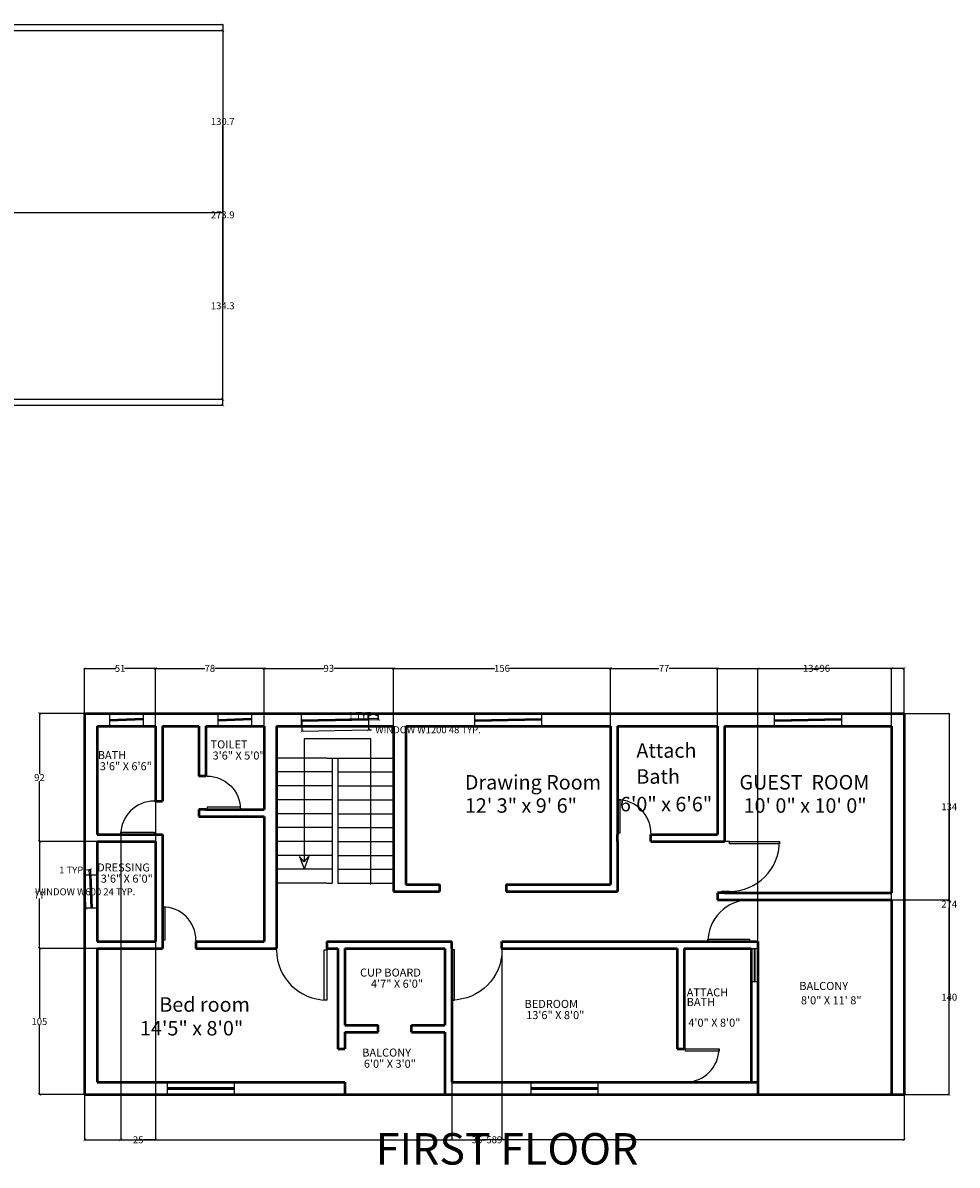
# Model space of a CAD drawing. Units: inches. Extents: x 1455 to 5994, y -182 to 2370.
# Tile 4 of 8: x 2291 to 2962, y 1415 to 2236. Entities that reach past the tile are written whole.
import ezdxf

# ---------------------------------------------------------------- set-up
doc = ezdxf.new("R2010")
doc.units = ezdxf.units.IN
doc.header["$MEASUREMENT"] = 0
doc.linetypes.add('CENTER', pattern=[50.8, 31.75, -6.35, 6.35, -6.35])
for name, color, linetype, lineweight in [('A-ANNO-DIMS', 2, 'Continuous', 18), ('A-ANNO-TEXT', 7, 'Continuous', 25), ('A-AREA-IDEN', 7, 'Continuous', 18), ('A-DOOR', 5, 'Continuous', 25), ('A-FLOR-STRS', 3, 'Continuous', 25), ('A-GLAZ', 4, 'Continuous', 25), ('A-GRID', 8, 'CENTER', 18), ('A-WALL', 7, 'Continuous', 50)]:
    doc.layers.add(name, color=color, linetype=linetype, lineweight=lineweight)
doc.styles.get("Standard").update_dxf_attribs({"font": 'arial.ttf'})
doc.dimstyles.get("Standard").update_dxf_attribs({"dimtxt": 5, "dimasz": 2, "dimexe": 0.18, "dimexo": 0.0625, "dimgap": 0.09, "dimtad": 0, "dimtih": 1, "dimtoh": 1, "dimdec": 1, "dimzin": 0, "dimdsep": 46, "dimlunit": 3, "dimtxsty": 'Standard', "dimblk": 'ARCHTICK', "dimcen": 0.09, "dimadec": 0, "dimazin": 0, "dimtfac": 1, "dimtdec": 1, "dimtofl": 0, "dimtmove": 0, "dimatfit": 3, "dimfxl": 1, "dimtolj": 1, "dimtzin": 0, "dimarcsym": 0})

# ---------------------------------------------------------------- blocks, each defined once
blk = doc.blocks.new('*U3')
for p, q in [((0, 0), (0, -6)), ((24, 0), (24, -6))]:
    blk.add_line(p, q)
blk.add_lwpolyline([(0, 0), (0, 24), (1.75, 24), (1.75, 0)], close=True)
blk.add_arc((0, 0), 24, 0, 90)
blk = doc.blocks.new('*U6')
for p, q in [((0, 0), (0, -6)), ((36, 0), (36, -6))]:
    blk.add_line(p, q)
blk.add_lwpolyline([(0, 0), (0, 36), (1.75, 36), (1.75, 0)], close=True)
blk.add_arc((0, 0), 36, 0, 90)
blk = doc.blocks.new('*U5')
for p, q in [((0, 0), (0, -6)), ((30, 0), (30, -6))]:
    blk.add_line(p, q)
blk.add_lwpolyline([(0, 0), (0, 30), (1.75, 30), (1.75, 0)], close=True)
blk.add_arc((0, 0), 30, 0, 90)
blk = doc.blocks.new('WIN-600')
for p, q in [((0, 0), (0, 24)), ((0.5, 0), (0.5, 24)), ((1, 0), (1, 24))]:
    blk.add_line(p, q)
blk = doc.blocks.new('WIN-1200')
for p, q in [((0, 1), (48, 1)), ((0, 0.5), (48, 0.5)), ((0, 0), (48, 0))]:
    blk.add_line(p, q)
blk = doc.blocks.new('WIN-1200-2L')
for p, q in [((0, 0.5), (48, 0.5)), ((0, 0), (48, 0))]:
    blk.add_line(p, q)
blk = doc.blocks.new('_ArchTick')
at = {"color": 0, "linetype": 'ByBlock', "const_width": 0.15}
blk.add_lwpolyline([(-0.5, -0.5), (0.5, 0.5)], dxfattribs=at)
blk = doc.blocks.new('*D21')
at = {"layer": 'A-ANNO-DIMS', "color": 0, "lineweight": -2, "transparency": 16777216}
for p, q in [((2338.59, 1623.65), (2334.88, 1623.5)), ((2335.06, 1623.51), (2335.45, 1614.19)), ((2336.06, 1599.53), (2335.67, 1608.84)), ((2339.59, 1599.67), (2335.88, 1599.52))]:
    blk.add_line(p, q, dxfattribs=at)
at = {"layer": 'Defpoints', "color": 0, "lineweight": 25, "transparency": 16777216}
for p in [(2338.66, 1623.65), (2336.06, 1599.53), (2339.65, 1599.68)]:
    blk.add_point(p, dxfattribs=at)
at = {"layer": 'A-ANNO-DIMS', "color": 0, "lineweight": -2, "transparency": 16777216, "xscale": 2, "yscale": 2, "zscale": 2}
for p, rotation in [((2335.06, 1623.51), 92.38594403038854), ((2336.06, 1599.53), 272.3859440303885)]:
    blk.add_blockref('_ArchTick', p, dxfattribs=dict(at, rotation=rotation))
at = {"layer": 'A-ANNO-DIMS', "color": 0, "transparency": 16777216, "insert": (2335.56, 1611.52), "char_height": 5, "attachment_point": 5}
blk.add_mtext('\\A1;WINDOW W600 24 TYP.', dxfattribs=at)
blk = doc.blocks.new('*D22')
at = {"layer": 'A-ANNO-DIMS', "color": 0, "lineweight": -2, "transparency": 16777216}
for p, q in [((2338.51, 1627.25), (2336.51, 1627.17)), ((2338.65, 1623.72), (2338.5, 1627.43)), ((2339.5, 1627.29), (2338.51, 1627.25)), ((2339.65, 1623.76), (2339.5, 1627.47))]:
    blk.add_line(p, q, dxfattribs=at)
at = {"layer": 'Defpoints', "color": 0, "lineweight": 25, "transparency": 16777216}
for p in [(2338.51, 1627.25), (2338.66, 1623.65), (2339.65, 1623.7)]:
    blk.add_point(p, dxfattribs=at)
at = {"layer": 'A-ANNO-DIMS', "color": 0, "lineweight": -2, "transparency": 16777216, "xscale": 2, "yscale": 2, "zscale": 2}
for p, rotation in [((2338.51, 1627.25), 182.385944030392), ((2339.5, 1627.29), 2.385944030392055)]:
    blk.add_blockref('_ArchTick', p, dxfattribs=dict(at, rotation=rotation))
at = {"layer": 'A-ANNO-DIMS', "color": 0, "transparency": 16777216, "insert": (2326.43, 1627.17), "char_height": 5, "attachment_point": 5}
blk.add_mtext('\\A1;1 TYP.', dxfattribs=at)
blk = doc.blocks.new('*D23')
at = {"layer": 'A-ANNO-DIMS', "color": 0, "lineweight": -2, "transparency": 16777216}
for p, q in [((2491.17, 1734.12), (2491.32, 1726.81)), ((2539.16, 1735.12), (2539.31, 1727.81)), ((2491.32, 1726.99), (2539.31, 1727.99)), ((2539.31, 1727.99), (2541.31, 1728.03))]:
    blk.add_line(p, q, dxfattribs=at)
at = {"layer": 'Defpoints', "color": 0, "lineweight": 25, "transparency": 16777216}
for p in [(2491.17, 1734.19), (2539.16, 1735.19), (2539.31, 1727.99)]:
    blk.add_point(p, dxfattribs=at)
at = {"layer": 'A-ANNO-DIMS', "color": 0, "lineweight": -2, "transparency": 16777216, "xscale": 2, "yscale": 2, "zscale": 2}
for p, rotation in [((2491.32, 1726.99), 181.1934894239818), ((2539.31, 1727.99), 1.193489423981775)]:
    blk.add_blockref('_ArchTick', p, dxfattribs=dict(at, rotation=rotation))
at = {"layer": 'A-ANNO-DIMS', "color": 0, "transparency": 16777216, "insert": (2582, 1728.03), "char_height": 5, "attachment_point": 5}
blk.add_mtext('\\A1;WINDOW W1200 48 TYP.', dxfattribs=at)
blk = doc.blocks.new('*D24')
at = {"layer": 'A-ANNO-DIMS', "color": 0, "lineweight": -2, "transparency": 16777216}
for p, q in [((2539.2, 1736.19), (2546.52, 1736.34)), ((2539.22, 1735.19), (2546.54, 1735.34)), ((2546.3, 1738.34), (2544.3, 1738.34)), ((2546.34, 1736.34), (2546.3, 1738.34)), ((2546.36, 1735.34), (2546.34, 1736.34))]:
    blk.add_line(p, q, dxfattribs=at)
at = {"layer": 'Defpoints', "color": 0, "lineweight": 25, "transparency": 16777216}
for p in [(2539.14, 1736.19), (2539.16, 1735.19), (2546.34, 1736.34)]:
    blk.add_point(p, dxfattribs=at)
at = {"layer": 'A-ANNO-DIMS', "color": 0, "lineweight": -2, "transparency": 16777216, "xscale": 2, "yscale": 2, "zscale": 2}
for p, rotation in [((2546.34, 1736.34), 91.19348942398422), ((2546.36, 1735.34), 271.1934894239842)]:
    blk.add_blockref('_ArchTick', p, dxfattribs=dict(at, rotation=rotation))
at = {"layer": 'A-ANNO-DIMS', "color": 0, "transparency": 16777216, "insert": (2534.21, 1738.34), "char_height": 5, "attachment_point": 5}
blk.add_mtext('\\A1;1 TYP.', dxfattribs=at)
blk = doc.blocks.new('*D39')
at = {"layer": 'A-ANNO-DIMS', "color": 0, "lineweight": -2, "transparency": 16777216}
for p, q in [((1483.73, 2230.77), (2434.6, 2230.77)), ((2434.42, 2230.77), (2434.42, 2168.07)), ((2434.42, 2100.07), (2434.42, 2162.78)), ((1484.89, 2100.07), (2434.6, 2100.07))]:
    blk.add_line(p, q, dxfattribs=at)
at = {"layer": 'Defpoints', "color": 0, "lineweight": 25, "transparency": 16777216}
for p in [(1483.66, 2230.77), (1484.83, 2100.07), (2434.42, 2100.07)]:
    blk.add_point(p, dxfattribs=at)
at = {"layer": 'A-ANNO-DIMS', "color": 0, "lineweight": -2, "transparency": 16777216, "xscale": 2, "yscale": 2, "zscale": 2}
for p, rotation in [((2434.42, 2230.77), 90), ((2434.42, 2100.07), 270)]:
    blk.add_blockref('_ArchTick', p, dxfattribs=dict(at, rotation=rotation))
at = {"layer": 'A-ANNO-DIMS', "color": 0, "transparency": 16777216, "insert": (2434.42, 2165.42), "char_height": 5, "attachment_point": 5}
blk.add_mtext('\\A1;130.7', dxfattribs=at)
blk = doc.blocks.new('*D40')
at = {"layer": 'A-ANNO-DIMS', "color": 0, "lineweight": -2, "transparency": 16777216}
for p, q in [((1484.89, 2100.07), (2434.6, 2100.07)), ((2434.42, 2100.07), (2434.42, 2035.57)), ((2434.42, 1965.77), (2434.42, 2030.28)), ((1483.73, 1965.77), (2434.6, 1965.77))]:
    blk.add_line(p, q, dxfattribs=at)
at = {"layer": 'Defpoints', "color": 0, "lineweight": 25, "transparency": 16777216}
for p in [(1484.83, 2100.07), (1483.66, 1965.77), (2434.42, 1965.77)]:
    blk.add_point(p, dxfattribs=at)
at = {"layer": 'A-ANNO-DIMS', "color": 0, "lineweight": -2, "transparency": 16777216, "xscale": 2, "yscale": 2, "zscale": 2}
for p, rotation in [((2434.42, 2100.07), 90), ((2434.42, 1965.77), 270)]:
    blk.add_blockref('_ArchTick', p, dxfattribs=dict(at, rotation=rotation))
at = {"layer": 'A-ANNO-DIMS', "color": 0, "transparency": 16777216, "insert": (2434.42, 2032.92), "char_height": 5, "attachment_point": 5}
blk.add_mtext('\\A1;134.3', dxfattribs=at)
blk = doc.blocks.new('*D42')
at = {"layer": 'A-ANNO-DIMS', "color": 0, "lineweight": -2, "transparency": 16777216}
for p, q in [((2177.86, 2235.27), (2434.6, 2235.27)), ((2434.42, 2235.27), (2434.42, 2100.96)), ((2434.42, 1961.36), (2434.42, 2095.67)), ((2177.86, 1961.36), (2434.6, 1961.36))]:
    blk.add_line(p, q, dxfattribs=at)
at = {"layer": 'Defpoints', "color": 0, "lineweight": 25, "transparency": 16777216}
for p in [(2177.79, 2235.27), (2434.42, 2235.27), (2177.79, 1961.36)]:
    blk.add_point(p, dxfattribs=at)
at = {"layer": 'A-ANNO-DIMS', "color": 0, "lineweight": -2, "transparency": 16777216, "xscale": 2, "yscale": 2, "zscale": 2}
for p, rotation in [((2434.42, 2235.27), 90), ((2434.42, 1961.36), 270)]:
    blk.add_blockref('_ArchTick', p, dxfattribs=dict(at, rotation=rotation))
at = {"layer": 'A-ANNO-DIMS', "color": 0, "transparency": 16777216, "insert": (2434.42, 2098.32), "char_height": 5, "attachment_point": 5}
blk.add_mtext('\\A1;273.9', dxfattribs=at)
blk = doc.blocks.new('*D68')
at = {"layer": 'A-ANNO-DIMS', "color": 0, "lineweight": -2, "transparency": 16777216}
for p, q in [((2335.15, 1465.62), (2335.15, 1433.01)), ((2924.15, 1465.62), (2924.15, 1433.01)), ((2335.15, 1433.19), (2624.04, 1433.19)), ((2924.15, 1433.19), (2635.27, 1433.19))]:
    blk.add_line(p, q, dxfattribs=at)
at = {"layer": 'Defpoints', "color": 0, "lineweight": 25, "transparency": 16777216}
for p in [(2335.15, 1465.69), (2924.15, 1465.69), (2924.15, 1433.19)]:
    blk.add_point(p, dxfattribs=at)
at = {"layer": 'A-ANNO-DIMS', "color": 0, "lineweight": -2, "transparency": 16777216, "xscale": 2, "yscale": 2, "zscale": 2, "rotation": 180}
blk.add_blockref('_ArchTick', (2335.15, 1433.19), dxfattribs=at)
at = {"layer": 'A-ANNO-DIMS', "color": 0, "lineweight": -2, "transparency": 16777216, "xscale": 2, "yscale": 2, "zscale": 2}
blk.add_blockref('_ArchTick', (2924.15, 1433.19), dxfattribs=at)
at = {"layer": 'A-ANNO-DIMS', "color": 0, "transparency": 16777216, "insert": (2629.65, 1433.19), "char_height": 5, "attachment_point": 5}
blk.add_mtext('\\A1;589', dxfattribs=at)
blk = doc.blocks.new('*D69')
at = {"layer": 'A-ANNO-DIMS', "color": 0, "lineweight": -2, "transparency": 16777216}
for p, q in [((2924.22, 1739.69), (2956.83, 1739.69)), ((2956.65, 1739.69), (2956.65, 1605.29)), ((2956.65, 1465.69), (2956.65, 1600.09)), ((2924.22, 1465.69), (2956.83, 1465.69))]:
    blk.add_line(p, q, dxfattribs=at)
at = {"layer": 'Defpoints', "color": 0, "lineweight": 25, "transparency": 16777216}
for p in [(2924.15, 1739.69), (2956.65, 1739.69), (2924.15, 1465.69)]:
    blk.add_point(p, dxfattribs=at)
at = {"layer": 'A-ANNO-DIMS', "color": 0, "lineweight": -2, "transparency": 16777216, "xscale": 2, "yscale": 2, "zscale": 2}
for p, rotation in [((2956.65, 1739.69), 90), ((2956.65, 1465.69), 270)]:
    blk.add_blockref('_ArchTick', p, dxfattribs=dict(at, rotation=rotation))
at = {"layer": 'A-ANNO-DIMS', "color": 0, "transparency": 16777216, "insert": (2956.65, 1602.69), "char_height": 5, "attachment_point": 5}
blk.add_mtext('\\A1;274', dxfattribs=at)
blk = doc.blocks.new('*D70')
at = {"layer": 'A-ANNO-DIMS', "color": 0, "lineweight": -2, "transparency": 16777216}
for p, q in [((2335.15, 1739.75), (2335.15, 1772.37)), ((2335.15, 1772.19), (2357.47, 1772.19)), ((2386.15, 1772.19), (2363.84, 1772.19)), ((2386.15, 1730.75), (2386.15, 1772.37))]:
    blk.add_line(p, q, dxfattribs=at)
at = {"layer": 'Defpoints', "color": 0, "lineweight": 25, "transparency": 16777216}
for p in [(2386.15, 1772.19), (2335.15, 1739.69), (2386.15, 1730.69)]:
    blk.add_point(p, dxfattribs=at)
at = {"layer": 'A-ANNO-DIMS', "color": 0, "lineweight": -2, "transparency": 16777216, "xscale": 2, "yscale": 2, "zscale": 2, "rotation": 180}
blk.add_blockref('_ArchTick', (2335.15, 1772.19), dxfattribs=at)
at = {"layer": 'A-ANNO-DIMS', "color": 0, "lineweight": -2, "transparency": 16777216, "xscale": 2, "yscale": 2, "zscale": 2}
blk.add_blockref('_ArchTick', (2386.15, 1772.19), dxfattribs=at)
at = {"layer": 'A-ANNO-DIMS', "color": 0, "transparency": 16777216, "insert": (2360.65, 1772.19), "char_height": 5, "attachment_point": 5}
blk.add_mtext('\\A1;51', dxfattribs=at)
blk = doc.blocks.new('*D71')
at = {"layer": 'A-ANNO-DIMS', "color": 0, "lineweight": -2, "transparency": 16777216}
for p, q in [((2386.15, 1730.75), (2386.15, 1772.37)), ((2386.15, 1772.19), (2421.5, 1772.19)), ((2464.15, 1772.19), (2428.81, 1772.19)), ((2464.15, 1730.75), (2464.15, 1772.37))]:
    blk.add_line(p, q, dxfattribs=at)
at = {"layer": 'Defpoints', "color": 0, "lineweight": 25, "transparency": 16777216}
for p in [(2464.15, 1772.19), (2386.15, 1730.69), (2464.15, 1730.69)]:
    blk.add_point(p, dxfattribs=at)
at = {"layer": 'A-ANNO-DIMS', "color": 0, "lineweight": -2, "transparency": 16777216, "xscale": 2, "yscale": 2, "zscale": 2, "rotation": 180}
blk.add_blockref('_ArchTick', (2386.15, 1772.19), dxfattribs=at)
at = {"layer": 'A-ANNO-DIMS', "color": 0, "lineweight": -2, "transparency": 16777216, "xscale": 2, "yscale": 2, "zscale": 2}
blk.add_blockref('_ArchTick', (2464.15, 1772.19), dxfattribs=at)
at = {"layer": 'A-ANNO-DIMS', "color": 0, "transparency": 16777216, "insert": (2425.15, 1772.19), "char_height": 5, "attachment_point": 5}
blk.add_mtext('\\A1;78', dxfattribs=at)
blk = doc.blocks.new('*D72')
at = {"layer": 'A-ANNO-DIMS', "color": 0, "lineweight": -2, "transparency": 16777216}
for p, q in [((2464.15, 1730.75), (2464.15, 1772.37)), ((2464.15, 1772.19), (2506.98, 1772.19)), ((2557.15, 1772.19), (2514.33, 1772.19)), ((2557.15, 1730.75), (2557.15, 1772.37))]:
    blk.add_line(p, q, dxfattribs=at)
at = {"layer": 'Defpoints', "color": 0, "lineweight": 25, "transparency": 16777216}
for p in [(2557.15, 1772.19), (2464.15, 1730.69), (2557.15, 1730.69)]:
    blk.add_point(p, dxfattribs=at)
at = {"layer": 'A-ANNO-DIMS', "color": 0, "lineweight": -2, "transparency": 16777216, "xscale": 2, "yscale": 2, "zscale": 2, "rotation": 180}
blk.add_blockref('_ArchTick', (2464.15, 1772.19), dxfattribs=at)
at = {"layer": 'A-ANNO-DIMS', "color": 0, "lineweight": -2, "transparency": 16777216, "xscale": 2, "yscale": 2, "zscale": 2}
blk.add_blockref('_ArchTick', (2557.15, 1772.19), dxfattribs=at)
at = {"layer": 'A-ANNO-DIMS', "color": 0, "transparency": 16777216, "insert": (2510.65, 1772.19), "char_height": 5, "attachment_point": 5}
blk.add_mtext('\\A1;93', dxfattribs=at)
blk = doc.blocks.new('*D73')
at = {"layer": 'A-ANNO-DIMS', "color": 0, "lineweight": -2, "transparency": 16777216}
for p, q in [((2557.15, 1730.75), (2557.15, 1772.37)), ((2557.15, 1772.19), (2629.78, 1772.19)), ((2713.15, 1772.19), (2640.53, 1772.19)), ((2713.15, 1730.75), (2713.15, 1772.37))]:
    blk.add_line(p, q, dxfattribs=at)
at = {"layer": 'Defpoints', "color": 0, "lineweight": 25, "transparency": 16777216}
for p in [(2713.15, 1772.19), (2557.15, 1730.69), (2713.15, 1730.69)]:
    blk.add_point(p, dxfattribs=at)
at = {"layer": 'A-ANNO-DIMS', "color": 0, "lineweight": -2, "transparency": 16777216, "xscale": 2, "yscale": 2, "zscale": 2, "rotation": 180}
blk.add_blockref('_ArchTick', (2557.15, 1772.19), dxfattribs=at)
at = {"layer": 'A-ANNO-DIMS', "color": 0, "lineweight": -2, "transparency": 16777216, "xscale": 2, "yscale": 2, "zscale": 2}
blk.add_blockref('_ArchTick', (2713.15, 1772.19), dxfattribs=at)
at = {"layer": 'A-ANNO-DIMS', "color": 0, "transparency": 16777216, "insert": (2635.15, 1772.19), "char_height": 5, "attachment_point": 5}
blk.add_mtext('\\A1;156', dxfattribs=at)
blk = doc.blocks.new('*D74')
at = {"layer": 'A-ANNO-DIMS', "color": 0, "lineweight": -2, "transparency": 16777216}
for p, q in [((2713.15, 1730.75), (2713.15, 1772.37)), ((2713.15, 1772.19), (2748, 1772.19)), ((2790.15, 1772.19), (2755.31, 1772.19)), ((2790.15, 1730.75), (2790.15, 1772.37))]:
    blk.add_line(p, q, dxfattribs=at)
at = {"layer": 'Defpoints', "color": 0, "lineweight": 25, "transparency": 16777216}
for p in [(2790.15, 1772.19), (2713.15, 1730.69), (2790.15, 1730.69)]:
    blk.add_point(p, dxfattribs=at)
at = {"layer": 'A-ANNO-DIMS', "color": 0, "lineweight": -2, "transparency": 16777216, "xscale": 2, "yscale": 2, "zscale": 2, "rotation": 180}
blk.add_blockref('_ArchTick', (2713.15, 1772.19), dxfattribs=at)
at = {"layer": 'A-ANNO-DIMS', "color": 0, "lineweight": -2, "transparency": 16777216, "xscale": 2, "yscale": 2, "zscale": 2}
blk.add_blockref('_ArchTick', (2790.15, 1772.19), dxfattribs=at)
at = {"layer": 'A-ANNO-DIMS', "color": 0, "transparency": 16777216, "insert": (2751.65, 1772.19), "char_height": 5, "attachment_point": 5}
blk.add_mtext('\\A1;77', dxfattribs=at)
blk = doc.blocks.new('*D75')
at = {"layer": 'A-ANNO-DIMS', "color": 0, "lineweight": -2, "transparency": 16777216}
for p, q in [((2790.15, 1730.75), (2790.15, 1772.37)), ((2790.15, 1772.19), (2851.79, 1772.19)), ((2924.15, 1772.19), (2862.52, 1772.19)), ((2924.15, 1739.75), (2924.15, 1772.37))]:
    blk.add_line(p, q, dxfattribs=at)
at = {"layer": 'Defpoints', "color": 0, "lineweight": 25, "transparency": 16777216}
for p in [(2924.15, 1772.19), (2924.15, 1739.69), (2790.15, 1730.69)]:
    blk.add_point(p, dxfattribs=at)
at = {"layer": 'A-ANNO-DIMS', "color": 0, "lineweight": -2, "transparency": 16777216, "xscale": 2, "yscale": 2, "zscale": 2, "rotation": 180}
blk.add_blockref('_ArchTick', (2790.15, 1772.19), dxfattribs=at)
at = {"layer": 'A-ANNO-DIMS', "color": 0, "lineweight": -2, "transparency": 16777216, "xscale": 2, "yscale": 2, "zscale": 2}
blk.add_blockref('_ArchTick', (2924.15, 1772.19), dxfattribs=at)
at = {"layer": 'A-ANNO-DIMS', "color": 0, "transparency": 16777216, "insert": (2857.15, 1772.19), "char_height": 5, "attachment_point": 5}
blk.add_mtext('\\A1;134', dxfattribs=at)
blk = doc.blocks.new('*D76')
at = {"layer": 'A-ANNO-DIMS', "color": 0, "lineweight": -2, "transparency": 16777216}
for p, q in [((2819.15, 1465.75), (2819.15, 1772.37)), ((2819.15, 1772.19), (2863.49, 1772.19)), ((2915.15, 1772.19), (2870.82, 1772.19)), ((2915.15, 1465.75), (2915.15, 1772.37))]:
    blk.add_line(p, q, dxfattribs=at)
at = {"layer": 'Defpoints', "color": 0, "lineweight": 25, "transparency": 16777216}
for p in [(2915.15, 1772.19), (2819.15, 1465.69), (2915.15, 1465.69)]:
    blk.add_point(p, dxfattribs=at)
at = {"layer": 'A-ANNO-DIMS', "color": 0, "lineweight": -2, "transparency": 16777216, "xscale": 2, "yscale": 2, "zscale": 2, "rotation": 180}
blk.add_blockref('_ArchTick', (2819.15, 1772.19), dxfattribs=at)
at = {"layer": 'A-ANNO-DIMS', "color": 0, "lineweight": -2, "transparency": 16777216, "xscale": 2, "yscale": 2, "zscale": 2}
blk.add_blockref('_ArchTick', (2915.15, 1772.19), dxfattribs=at)
at = {"layer": 'A-ANNO-DIMS', "color": 0, "transparency": 16777216, "insert": (2867.15, 1772.19), "char_height": 5, "attachment_point": 5}
blk.add_mtext('\\A1;96', dxfattribs=at)
blk = doc.blocks.new('*D77')
at = {"layer": 'A-ANNO-DIMS', "color": 0, "lineweight": -2, "transparency": 16777216}
for p, q in [((2344.09, 1570.69), (2302.47, 1570.69)), ((2302.65, 1570.69), (2302.65, 1520.83)), ((2302.65, 1465.69), (2302.65, 1515.54)), ((2335.09, 1465.69), (2302.47, 1465.69))]:
    blk.add_line(p, q, dxfattribs=at)
at = {"layer": 'Defpoints', "color": 0, "lineweight": 25, "transparency": 16777216}
for p in [(2302.65, 1570.69), (2344.15, 1570.69), (2335.15, 1465.69)]:
    blk.add_point(p, dxfattribs=at)
at = {"layer": 'A-ANNO-DIMS', "color": 0, "lineweight": -2, "transparency": 16777216, "xscale": 2, "yscale": 2, "zscale": 2}
for p, rotation in [((2302.65, 1570.69), 90), ((2302.65, 1465.69), 270)]:
    blk.add_blockref('_ArchTick', p, dxfattribs=dict(at, rotation=rotation))
at = {"layer": 'A-ANNO-DIMS', "color": 0, "transparency": 16777216, "insert": (2302.65, 1518.19), "char_height": 5, "attachment_point": 5}
blk.add_mtext('\\A1;105', dxfattribs=at)
blk = doc.blocks.new('*D78')
at = {"layer": 'A-ANNO-DIMS', "color": 0, "lineweight": -2, "transparency": 16777216}
for p, q in [((2344.092084, 1647.686089), (2302.474584, 1647.686089)), ((2302.654584, 1647.686089), (2302.654584, 1611.776089)), ((2302.654584, 1570.686089), (2302.654584, 1606.596089)), ((2344.092084, 1570.686089), (2302.474584, 1570.686089))]:
    blk.add_line(p, q, dxfattribs=at)
at = {"layer": 'Defpoints', "color": 0, "lineweight": 25, "transparency": 16777216}
for p in [(2302.654584, 1647.686089), (2344.154584, 1647.686089), (2344.154584, 1570.686089)]:
    blk.add_point(p, dxfattribs=at)
at = {"layer": 'A-ANNO-DIMS', "color": 0, "lineweight": -2, "transparency": 16777216, "xscale": 2, "yscale": 2, "zscale": 2}
for p, rotation in [((2302.654584, 1647.686089), 90), ((2302.654584, 1570.686089), 270)]:
    blk.add_blockref('_ArchTick', p, dxfattribs=dict(at, rotation=rotation))
at = {"layer": 'A-ANNO-DIMS', "color": 0, "transparency": 16777216, "insert": (2302.654584, 1609.186089), "char_height": 5, "attachment_point": 5}
blk.add_mtext('\\A1;77', dxfattribs=at)
blk = doc.blocks.new('*D79')
at = {"layer": 'A-ANNO-DIMS', "color": 0, "lineweight": -2, "transparency": 16777216}
for p, q in [((2335.09, 1739.69), (2302.47, 1739.69)), ((2302.65, 1739.69), (2302.65, 1696.33)), ((2302.65, 1647.69), (2302.65, 1691.04)), ((2344.09, 1647.69), (2302.47, 1647.69))]:
    blk.add_line(p, q, dxfattribs=at)
at = {"layer": 'Defpoints', "color": 0, "lineweight": 25, "transparency": 16777216}
for p in [(2302.65, 1739.69), (2335.15, 1739.69), (2344.15, 1647.69)]:
    blk.add_point(p, dxfattribs=at)
at = {"layer": 'A-ANNO-DIMS', "color": 0, "lineweight": -2, "transparency": 16777216, "xscale": 2, "yscale": 2, "zscale": 2}
for p, rotation in [((2302.65, 1739.69), 90), ((2302.65, 1647.69), 270)]:
    blk.add_blockref('_ArchTick', p, dxfattribs=dict(at, rotation=rotation))
at = {"layer": 'A-ANNO-DIMS', "color": 0, "transparency": 16777216, "insert": (2302.65, 1693.69), "char_height": 5, "attachment_point": 5}
blk.add_mtext('\\A1;92', dxfattribs=at)
blk = doc.blocks.new('*D80')
at = {"layer": 'A-ANNO-DIMS', "color": 0, "lineweight": -2, "transparency": 16777216}
for p, q in [((2915.22, 1605.69), (2956.83, 1605.69)), ((2956.65, 1605.69), (2956.65, 1538.33)), ((2956.65, 1465.69), (2956.65, 1533.04)), ((2924.22, 1465.69), (2956.83, 1465.69))]:
    blk.add_line(p, q, dxfattribs=at)
at = {"layer": 'Defpoints', "color": 0, "lineweight": 25, "transparency": 16777216}
for p in [(2915.15, 1605.69), (2956.65, 1605.69), (2924.15, 1465.69)]:
    blk.add_point(p, dxfattribs=at)
at = {"layer": 'A-ANNO-DIMS', "color": 0, "lineweight": -2, "transparency": 16777216, "xscale": 2, "yscale": 2, "zscale": 2}
for p, rotation in [((2956.65, 1605.69), 90), ((2956.65, 1465.69), 270)]:
    blk.add_blockref('_ArchTick', p, dxfattribs=dict(at, rotation=rotation))
at = {"layer": 'A-ANNO-DIMS', "color": 0, "transparency": 16777216, "insert": (2956.65, 1535.69), "char_height": 5, "attachment_point": 5}
blk.add_mtext('\\A1;140', dxfattribs=at)
blk = doc.blocks.new('*D81')
at = {"layer": 'A-ANNO-DIMS', "color": 0, "lineweight": -2, "transparency": 16777216}
for p, q in [((2924.22, 1739.69), (2956.83, 1739.69)), ((2956.65, 1739.69), (2956.65, 1675.33)), ((2956.65, 1605.69), (2956.65, 1670.04)), ((2915.22, 1605.69), (2956.83, 1605.69))]:
    blk.add_line(p, q, dxfattribs=at)
at = {"layer": 'Defpoints', "color": 0, "lineweight": 25, "transparency": 16777216}
for p in [(2924.15, 1739.69), (2956.65, 1739.69), (2915.15, 1605.69)]:
    blk.add_point(p, dxfattribs=at)
at = {"layer": 'A-ANNO-DIMS', "color": 0, "lineweight": -2, "transparency": 16777216, "xscale": 2, "yscale": 2, "zscale": 2}
for p, rotation in [((2956.65, 1739.69), 90), ((2956.65, 1605.69), 270)]:
    blk.add_blockref('_ArchTick', p, dxfattribs=dict(at, rotation=rotation))
at = {"layer": 'A-ANNO-DIMS', "color": 0, "transparency": 16777216, "insert": (2956.65, 1672.69), "char_height": 5, "attachment_point": 5}
blk.add_mtext('\\A1;134', dxfattribs=at)
blk = doc.blocks.new('*D82')
at = {"layer": 'A-ANNO-DIMS', "color": 0, "lineweight": -2, "transparency": 16777216}
for p, q in [((2599.15, 1575.62), (2599.15, 1433.01)), ((2635.15, 1575.62), (2635.15, 1433.01)), ((2599.15, 1433.19), (2613.49, 1433.19)), ((2635.15, 1433.19), (2620.82, 1433.19))]:
    blk.add_line(p, q, dxfattribs=at)
at = {"layer": 'Defpoints', "color": 0, "lineweight": 25, "transparency": 16777216}
for p in [(2599.15, 1575.69), (2635.15, 1575.69), (2635.15, 1433.19)]:
    blk.add_point(p, dxfattribs=at)
at = {"layer": 'A-ANNO-DIMS', "color": 0, "lineweight": -2, "transparency": 16777216, "xscale": 2, "yscale": 2, "zscale": 2, "rotation": 180}
blk.add_blockref('_ArchTick', (2599.15, 1433.19), dxfattribs=at)
at = {"layer": 'A-ANNO-DIMS', "color": 0, "lineweight": -2, "transparency": 16777216, "xscale": 2, "yscale": 2, "zscale": 2}
blk.add_blockref('_ArchTick', (2635.15, 1433.19), dxfattribs=at)
at = {"layer": 'A-ANNO-DIMS', "color": 0, "transparency": 16777216, "insert": (2617.15, 1433.19), "char_height": 5, "attachment_point": 5}
blk.add_mtext('\\A1;36', dxfattribs=at)
blk = doc.blocks.new('*D83')
at = {"layer": 'A-ANNO-DIMS', "color": 0, "lineweight": -2, "transparency": 16777216}
for p, q in [((2386.15, 1676.62), (2386.15, 1433.01)), ((2361.15, 1652.62), (2361.15, 1433.01)), ((2361.15, 1433.19), (2369.92, 1433.19)), ((2386.15, 1433.19), (2377.39, 1433.19))]:
    blk.add_line(p, q, dxfattribs=at)
at = {"layer": 'Defpoints', "color": 0, "lineweight": 25, "transparency": 16777216}
for p in [(2386.15, 1676.69), (2361.15, 1652.69), (2386.15, 1433.19)]:
    blk.add_point(p, dxfattribs=at)
at = {"layer": 'A-ANNO-DIMS', "color": 0, "lineweight": -2, "transparency": 16777216, "xscale": 2, "yscale": 2, "zscale": 2, "rotation": 180}
blk.add_blockref('_ArchTick', (2361.15, 1433.19), dxfattribs=at)
at = {"layer": 'A-ANNO-DIMS', "color": 0, "lineweight": -2, "transparency": 16777216, "xscale": 2, "yscale": 2, "zscale": 2}
blk.add_blockref('_ArchTick', (2386.15, 1433.19), dxfattribs=at)
at = {"layer": 'A-ANNO-DIMS', "color": 0, "transparency": 16777216, "insert": (2373.65, 1433.19), "char_height": 5, "attachment_point": 5}
blk.add_mtext('\\A1;25', dxfattribs=at)

msp = doc.modelspace()

# ---------------------------------------------------------------- linework, layer by layer
at = {"layer": 'A-FLOR-STRS'}
for p, q in [((2540.9796, 1721.5573), (2492.9796, 1721.5573)), ((2492.9796, 1721.5573), (2492.9796, 1632.9997)), ((2540.9796, 1616.8618), (2540.9796, 1721.5573)), ((2509.1546, 1707.6861), (2473.1546, 1707.6861)), ((2509.1546, 1707.6861), (2521.1546, 1707.6861)), ((2513.1546, 1707.6861), (2513.1546, 1617.6861)), ((2517.1546, 1707.6861), (2517.1546, 1617.6861)), ((2521.1546, 1707.6861), (2557.1546, 1707.6861)), ((2513.1546, 1697.6861), (2473.1546, 1697.6861)), ((2517.1546, 1697.6861), (2557.1546, 1697.6861)), ((2513.1546, 1687.6861), (2473.1546, 1687.6861)), ((2517.1546, 1687.6861), (2557.1546, 1687.6861)), ((2513.1546, 1677.6861), (2473.1546, 1677.6861)), ((2517.1546, 1677.6861), (2557.1546, 1677.6861)), ((2513.1546, 1667.6861), (2473.1546, 1667.6861)), ((2517.1546, 1667.6861), (2557.1546, 1667.6861)), ((2513.1546, 1657.6861), (2473.1546, 1657.6861)), ((2517.1546, 1657.6861), (2557.1546, 1657.6861)), ((2513.1546, 1647.6861), (2473.1546, 1647.6861)), ((2517.1546, 1647.6861), (2557.1546, 1647.6861)), ((2513.1546, 1637.6861), (2473.1546, 1637.6861)), ((2492.9796, 1632.9997), (2489.632, 1636.8618)), ((2489.632, 1636.8618), (2492.9796, 1627.9809)), ((2492.9796, 1632.9997), (2496.3273, 1636.8618)), ((2496.3273, 1636.8618), (2492.9796, 1627.9809)), ((2517.1546, 1637.6861), (2557.1546, 1637.6861)), ((2513.1546, 1627.6861), (2473.1546, 1627.6861)), ((2517.1546, 1627.6861), (2557.1546, 1627.6861)), ((2509.1546, 1617.6861), (2473.1546, 1617.6861)), ((2509.1546, 1617.6861), (2513.1546, 1617.6861)), ((2517.1546, 1617.6861), (2521.1546, 1617.6861)), ((2521.1546, 1617.6861), (2557.1546, 1617.6861))]:
    msp.add_line(p, q, dxfattribs=at)
at = {"layer": 'A-GLAZ'}
for p, q in [((2816.4546, 1570.6861), (2816.4546, 1546.6861)), ((2816.8546, 1570.6861), (2816.8546, 1546.6861)), ((2394.6546, 1469.6861), (2442.6546, 1469.6861)), ((2656.1546, 1469.6861), (2704.1546, 1469.6861))]:
    msp.add_line(p, q, dxfattribs=at)
for points in [[(2353.1546, 1739.6861), (2377.1546, 1739.6861), (2377.1546, 1730.6861), (2353.1546, 1730.6861)], [(2431.1546, 1739.6861), (2455.1546, 1739.6861), (2455.1546, 1730.6861), (2431.1546, 1730.6861)], [(2491.1546, 1739.6861), (2539.1546, 1739.6861), (2539.1546, 1730.6861), (2491.1546, 1730.6861)], [(2615.6546, 1739.6861), (2663.6546, 1739.6861), (2663.6546, 1730.6861), (2615.6546, 1730.6861)], [(2831.1546, 1739.6861), (2879.1546, 1739.6861), (2879.1546, 1730.6861), (2831.1546, 1730.6861)], [(2335.1546, 1599.6861), (2335.1546, 1623.6861), (2344.1546, 1623.6861), (2344.1546, 1599.6861)], [(2819.1546, 1546.6861), (2814.1546, 1546.6861), (2814.1546, 1570.6861), (2819.1546, 1570.6861)], [(2394.6546, 1474.6861), (2442.6546, 1474.6861), (2442.6546, 1465.6861), (2394.6546, 1465.6861)], [(2656.1546, 1474.6861), (2704.1546, 1474.6861), (2704.1546, 1465.6861), (2656.1546, 1465.6861)]]:
    msp.add_lwpolyline(points, close=True, dxfattribs=at)
at = {"layer": 'A-GRID'}
msp.add_line((1483.6636, 1965.774), (2386.1674, 1965.774), dxfattribs=at)
at = {"layer": 'A-WALL'}
for p, q in [((2335.1546, 1739.6861), (2335.1546, 1465.6861)), ((2335.1546, 1739.6861), (2924.1546, 1739.6861)), ((2924.1546, 1739.6861), (2924.1546, 1465.6861)), ((2344.1546, 1730.6861), (2344.1546, 1652.6861)), ((2344.1546, 1730.6861), (2386.1546, 1730.6861)), ((2386.1546, 1730.6861), (2386.1546, 1676.6861)), ((2391.1546, 1730.6861), (2391.1546, 1676.6861)), ((2391.1546, 1730.6861), (2417.1546, 1730.6861)), ((2417.1546, 1730.6861), (2417.1546, 1694.6861)), ((2422.1546, 1730.6861), (2422.1546, 1694.6861)), ((2422.1546, 1730.6861), (2464.1546, 1730.6861)), ((2464.1546, 1730.6861), (2464.1546, 1670.6861)), ((2473.1546, 1730.6861), (2473.1546, 1575.6861)), ((2473.1546, 1730.6861), (2557.1546, 1730.6861)), ((2557.1546, 1730.6861), (2557.1546, 1611.6861)), ((2566.1546, 1730.6861), (2566.1546, 1616.6861)), ((2566.1546, 1730.6861), (2713.1546, 1730.6861)), ((2713.1546, 1730.6861), (2713.1546, 1616.6861)), ((2718.1546, 1730.6861), (2718.1546, 1652.6861)), ((2718.1546, 1730.6861), (2790.1546, 1730.6861)), ((2790.1546, 1730.6861), (2790.1546, 1652.6861)), ((2795.1546, 1730.6861), (2795.1546, 1647.6861)), ((2795.1546, 1730.6861), (2915.1546, 1730.6861)), ((2915.1546, 1730.6861), (2915.1546, 1610.6861)), ((2422.1546, 1694.6861), (2417.1546, 1694.6861)), ((2386.1546, 1676.6861), (2391.1546, 1676.6861)), ((2422.1546, 1670.6861), (2417.1546, 1670.6861)), ((2417.1546, 1670.6861), (2417.1546, 1665.6861)), ((2422.1546, 1670.6861), (2464.1546, 1670.6861)), ((2417.1546, 1665.6861), (2464.1546, 1665.6861)), ((2464.1546, 1665.6861), (2464.1546, 1575.6861)), ((2344.1546, 1652.6861), (2386.1546, 1652.6861)), ((2386.1546, 1652.6861), (2391.1546, 1652.6861)), ((2391.1546, 1652.6861), (2391.1546, 1575.6861)), ((2718.1546, 1647.6861), (2718.1546, 1652.6861)), ((2742.1546, 1652.6861), (2790.1546, 1652.6861)), ((2742.1546, 1647.6861), (2742.1546, 1652.6861)), ((2344.1546, 1647.6861), (2386.1546, 1647.6861)), ((2344.1546, 1647.6861), (2344.1546, 1575.6861)), ((2386.1546, 1647.6861), (2386.1546, 1575.6861)), ((2718.1546, 1647.6861), (2718.1546, 1611.6861)), ((2742.1546, 1647.6861), (2790.1546, 1647.6861)), ((2790.1546, 1647.6861), (2795.1546, 1647.6861)), ((2557.1546, 1611.6861), (2590.1546, 1611.6861)), ((2566.1546, 1616.6861), (2590.1546, 1616.6861)), ((2590.1546, 1616.6861), (2590.1546, 1611.6861)), ((2638.1546, 1616.6861), (2638.1546, 1611.6861)), ((2638.1546, 1616.6861), (2713.1546, 1616.6861)), ((2638.1546, 1611.6861), (2718.1546, 1611.6861)), ((2790.1546, 1610.6861), (2790.1546, 1605.6861)), ((2795.1546, 1610.6861), (2790.1546, 1610.6861)), ((2795.1546, 1610.6861), (2915.1546, 1610.6861)), ((2790.1546, 1605.6861), (2915.1546, 1605.6861)), ((2915.1546, 1605.6861), (2915.1546, 1465.6861)), ((2344.1546, 1575.6861), (2386.1546, 1575.6861)), ((2344.1546, 1570.6861), (2391.1546, 1570.6861)), ((2344.1546, 1570.6861), (2344.1546, 1474.6861)), ((2391.1546, 1575.6861), (2391.1546, 1570.6861)), ((2415.1546, 1575.6861), (2415.1546, 1570.6861)), ((2415.1546, 1575.6861), (2422.1546, 1575.6861)), ((2415.1546, 1570.6861), (2473.1546, 1570.6861)), ((2422.1546, 1575.6861), (2464.1546, 1575.6861)), ((2473.1546, 1575.6861), (2473.1546, 1570.6861)), ((2509.1546, 1575.6861), (2566.1546, 1575.6861)), ((2509.1546, 1575.6861), (2509.1546, 1570.6861)), ((2509.1546, 1570.6861), (2517.1546, 1570.6861)), ((2517.1546, 1570.6861), (2517.1546, 1498.6861)), ((2522.1546, 1570.6861), (2522.1546, 1515.6861)), ((2522.1546, 1570.6861), (2594.1546, 1570.6861)), ((2566.1546, 1575.6861), (2599.1546, 1575.6861)), ((2575.1546, 1570.6861), (2594.1546, 1570.6861)), ((2594.1546, 1570.6861), (2594.1546, 1515.6861)), ((2599.1546, 1570.6861), (2599.1546, 1575.6861)), ((2599.1546, 1570.6861), (2599.1546, 1474.6861)), ((2635.1546, 1570.6861), (2635.1546, 1575.6861)), ((2635.1546, 1575.6861), (2819.1546, 1575.6861)), ((2635.1546, 1570.6861), (2761.1546, 1570.6861)), ((2761.1546, 1570.6861), (2761.1546, 1498.6861)), ((2766.1546, 1570.6861), (2766.1546, 1498.6861)), ((2766.1546, 1570.6861), (2814.1546, 1570.6861)), ((2790.1546, 1570.6861), (2795.1546, 1570.6861)), ((2814.1546, 1570.6861), (2814.1546, 1474.6861)), ((2819.1546, 1575.6861), (2819.1546, 1465.6861)), ((2522.1546, 1515.6861), (2546.1546, 1515.6861)), ((2546.1546, 1510.6861), (2546.1546, 1515.6861)), ((2570.1546, 1510.6861), (2570.1546, 1515.6861)), ((2570.1546, 1515.6861), (2594.1546, 1515.6861)), ((2522.1546, 1510.6861), (2546.1546, 1510.6861)), ((2522.1546, 1510.6861), (2522.1546, 1498.6861)), ((2570.1546, 1510.6861), (2594.1546, 1510.6861)), ((2594.1546, 1510.6861), (2594.1546, 1474.6861)), ((2517.1546, 1498.6861), (2522.1546, 1498.6861)), ((2761.1546, 1498.6861), (2766.1546, 1498.6861)), ((2344.1546, 1474.6861), (2493.1546, 1474.6861)), ((2493.1546, 1474.6861), (2517.1546, 1474.6861)), ((2517.1546, 1474.6861), (2522.1546, 1474.6861)), ((2522.1546, 1474.6861), (2522.1546, 1465.6861)), ((2594.1546, 1474.6861), (2594.1546, 1465.6861)), ((2599.1546, 1474.6861), (2761.1546, 1474.6861)), ((2761.1546, 1474.6861), (2766.1546, 1474.6861)), ((2766.1546, 1474.6861), (2819.1546, 1474.6861)), ((2335.1546, 1465.6861), (2924.1546, 1465.6861))]:
    msp.add_line(p, q, dxfattribs=at)

# ---------------------------------------------------------------- block references
at = {"layer": 'A-DOOR', "xscale": -1}
for name, p, rotation in [('*U3', (2423.1546, 1670.6861), 270), ('*U6', (2599.1546, 1569.6861), 180)]:
    msp.add_blockref(name, p, dxfattribs=dict(at, rotation=rotation))
at = {"layer": 'A-DOOR'}
for name, p, rotation in [('*U3', (2385.1546, 1652.6861), 90), ('*U6', (2798.6546, 1647.6861), 270), ('*U5', (2813.1546, 1575.6861), 90), ('*U6', (2509.1546, 1569.6861), 180), ('*U3', (2767.1546, 1498.6861), 270)]:
    msp.add_blockref(name, p, dxfattribs=dict(at, rotation=rotation))
for p in [(2718.1546, 1653.6861), (2391.1546, 1576.6861)]:
    msp.add_blockref('*U3', p, dxfattribs=at)
at = {"layer": 'A-GLAZ'}
for name, p, rotation in [('WIN-600', (2377.1651, 1735.1866), 92.3859440303877), ('WIN-600', (2455.1651, 1735.1866), 92.3859440303877), ('WIN-1200', (2491.1707, 1734.1862), 1.193489423981743), ('WIN-1200', (2615.6707, 1734.1862), 1.193489423981743), ('WIN-1200', (2831.1707, 1734.1862), 1.193489423981743), ('WIN-600', (2339.6541, 1623.6966), 182.3859440303887)]:
    msp.add_blockref(name, p, dxfattribs=dict(at, rotation=rotation))
for p in [(2394.655, 1470.186), (2656.155, 1470.186)]:
    msp.add_blockref('WIN-1200-2L', p, dxfattribs=at)

# ---------------------------------------------------------------- texts
at = {"layer": 'A-ANNO-TEXT'}
msp.add_text('FIRST FLOOR', height=22.629125, dxfattribs=at).set_placement((2544.465, 1415.3353))
at = {"layer": 'A-AREA-IDEN'}
for s, height, p in [('TOILET', 5.78042, (2425.6713, 1714.6291)), ('Attach', 10.41336, (2731.7381, 1707.9189)), ('BATH', 5.78042, (2344.595, 1706.9384)), ('3\'6" X 5\'0"', 5.780423, (2427.1152, 1706.6002)), ('3\'6" X 6\'6"', 5.780423, (2346.0389, 1698.9095)), ('Bath', 10.41336, (2731.7381, 1689.2391)), ('Drawing Room', 10.413361, (2608.4755, 1685.0676)), ('GUEST  ROOM', 10.413361, (2805.8408, 1685.0676)), ('12\' 3" x 9\' 6"', 10.413361, (2608.4755, 1668.3395)), ('6\'0" x 6\'6"', 10.413361, (2719.9046, 1669.3555)), ('10\' 0" x 10\' 0"', 10.413361, (2808.8161, 1668.3395)), ('DRESSING', 5.78042, (2344.1546, 1626.119)), ('3\'6" X 6\'0"', 5.780423, (2346.7498, 1618.0901)), ('CUP BOARD', 5.78042, (2533.1353, 1550.5372)), ('4\'7" X 6\'0"', 5.780423, (2540.9952, 1542.5083)), ('BALCONY', 5.78042, (2848.9084, 1540.9038)), ('Bed room', 10.41336, (2388.8499, 1525.2561)), ('ATTACH', 5.78042, (2767.9437, 1536.2756)), ('8\'0" X 11\' 8"', 5.780423, (2850.0619, 1530.578)), ('BEDROOM', 5.78042, (2651.3981, 1527.9846)), ('BATH', 5.78042, (2767.9437, 1529.3719)), ('13\'6" X 8\'0"', 5.780423, (2652.5516, 1519.9557)), ('4\'0" X 8\'0"', 5.780423, (2769.0972, 1514.5052)), ('14\'5" x 8\'0"', 10.413361, (2374.9592, 1508.1884)), ('BALCONY', 5.78042, (2534.7081, 1492.9947)), ('6\'0" X 3\'0"', 5.780423, (2535.8615, 1484.9658))]:
    msp.add_text(s, height=height, dxfattribs=at).set_placement(p)

# ---------------------------------------------------------------- dimensions: what is measured, and where the dimension line sits
at = {"layer": 'A-ANNO-DIMS'}
for base, p1, p2, override, picture, middle in [((2434.4174, 2235.274), (2177.7942, 1961.3596), (2177.7942, 2235.274), {"dimdec": 1, "dimlfac": 1, "dimrnd": 0, "dimzin": 0, "dimdsep": 46, "dimlunit": 2}, '*D42', (2434.4174, 2098.3168)), ((2434.4174, 2100.0669), (1483.6636, 2230.774), (1484.8312, 2100.0669), {"dimdec": 1, "dimlfac": 1, "dimrnd": 0, "dimzin": 0, "dimdsep": 46, "dimlunit": 2}, '*D39', (2434.4174, 2165.4205)), ((2434.4174, 1965.774), (1484.8312, 2100.0669), (1483.6636, 1965.774), {"dimdec": 1, "dimlfac": 1, "dimrnd": 0, "dimzin": 0, "dimdsep": 46, "dimlunit": 2}, '*D40', (2434.4174, 2032.9205)), ((2302.6546, 1739.6861), (2344.1546, 1647.6861), (2335.1546, 1739.6861), {"dimdec": 0, "dimlfac": 1, "dimrnd": 0, "dimzin": 0, "dimdsep": 46, "dimlunit": 2}, '*D79', (2302.6546, 1693.6861)), ((2956.6546, 1739.6861), (2915.1546, 1605.6861), (2924.1546, 1739.6861), {"dimdec": 0, "dimlfac": 1, "dimrnd": 0, "dimzin": 0, "dimdsep": 46, "dimlunit": 2}, '*D81', (2956.6546, 1672.6861)), ((2956.6546, 1739.6861), (2924.1546, 1465.6861), (2924.1546, 1739.6861), {"dimdec": 0, "dimlfac": 1, "dimrnd": 0, "dimzin": 0, "dimdsep": 46, "dimlunit": 2}, '*D69', (2956.6546, 1602.6861)), ((2302.6546, 1647.6861), (2344.1546, 1570.6861), (2344.1546, 1647.6861), {"dimdec": 0, "dimlfac": 1, "dimrnd": 0, "dimzin": 0, "dimdsep": 46, "dimlunit": 2}, '*D78', (2302.6546, 1609.1861)), ((2956.6546, 1605.6861), (2924.1546, 1465.6861), (2915.1546, 1605.6861), {"dimdec": 0, "dimlfac": 1, "dimrnd": 0, "dimzin": 0, "dimdsep": 46, "dimlunit": 2}, '*D80', (2956.6546, 1535.6861)), ((2302.6546, 1570.6861), (2335.1546, 1465.6861), (2344.1546, 1570.6861), {"dimdec": 0, "dimlfac": 1, "dimrnd": 0, "dimzin": 0, "dimdsep": 46, "dimlunit": 2}, '*D77', (2302.6546, 1518.1861))]:
    dim = msp.add_linear_dim(base=base, p1=p1, p2=p2, angle=90, dimstyle='Standard', override=override, dxfattribs=at)
    dim.commit()
    dim.dimension.update_dxf_attribs({"geometry": picture, "text_midpoint": middle})
for base, p1, p2, picture, middle in [((2386.1546, 1772.1861), (2335.1546, 1739.6861), (2386.1546, 1730.6861), '*D70', (2360.6546, 1772.1861)), ((2464.1546, 1772.1861), (2386.1546, 1730.6861), (2464.1546, 1730.6861), '*D71', (2425.1546, 1772.1861)), ((2557.1546, 1772.1861), (2464.1546, 1730.6861), (2557.1546, 1730.6861), '*D72', (2510.6546, 1772.1861)), ((2713.1546, 1772.1861), (2557.1546, 1730.6861), (2713.1546, 1730.6861), '*D73', (2635.1546, 1772.1861)), ((2790.1546, 1772.1861), (2713.1546, 1730.6861), (2790.1546, 1730.6861), '*D74', (2751.6546, 1772.1861)), ((2924.1546, 1772.1861), (2790.1546, 1730.6861), (2924.1546, 1739.6861), '*D75', (2857.1546, 1772.1861)), ((2915.1546, 1772.1861), (2819.1546, 1465.6861), (2915.1546, 1465.6861), '*D76', (2867.1546, 1772.1861)), ((2386.1546, 1433.1861), (2361.1546, 1652.6861), (2386.1546, 1676.6861), '*D83', (2373.6546, 1433.1861)), ((2635.1546, 1433.1861), (2599.1546, 1575.6861), (2635.1546, 1575.6861), '*D82', (2617.1546, 1433.1861)), ((2924.1546, 1433.1861), (2335.1546, 1465.6861), (2924.1546, 1465.6861), '*D68', (2629.6546, 1433.1861))]:
    dim = msp.add_linear_dim(base=base, p1=p1, p2=p2, dimstyle='Standard', override={"dimdec": 0, "dimlfac": 1, "dimrnd": 0, "dimzin": 0, "dimdsep": 46, "dimlunit": 2}, dxfattribs=at)
    dim.commit()
    dim.dimension.update_dxf_attribs({"geometry": picture, "text_midpoint": middle})
for base, p1, p2, angle, text, picture, middle in [((2539.3098, 1727.9877), (2491.1702, 1734.1863), (2539.1598, 1735.1861), 1.1934894, 'WINDOW W1200 <> TYP.', '*D23', (2582.0013, 1728.0293)), ((2546.3374, 1736.3358), (2539.1598, 1735.1861), (2539.139, 1736.1859), 91.1934894, '<> TYP.', '*D24', (2534.2143, 1738.3354)), ((2336.0577, 1599.5258), (2338.6555, 1623.6549), (2339.6546, 1599.6757), 272.385944, 'WINDOW W600 <> TYP.', '*D21', (2335.5581, 1611.5154)), ((2338.5056, 1627.2517), (2339.6546, 1623.6965), (2338.6555, 1623.6549), 182.385944, '<> TYP.', '*D22', (2326.4258, 1627.1685))]:
    dim = msp.add_linear_dim(base=base, p1=p1, p2=p2, angle=angle, text=text, dimstyle='Standard', override={"dimdec": 0, "dimlfac": 1, "dimrnd": 0, "dimzin": 0, "dimdsep": 46, "dimlunit": 2}, dxfattribs=at)
    dim.commit()
    dim.dimension.update_dxf_attribs({"geometry": picture, "text_midpoint": middle})

doc.saveas('drawing.dxf')
